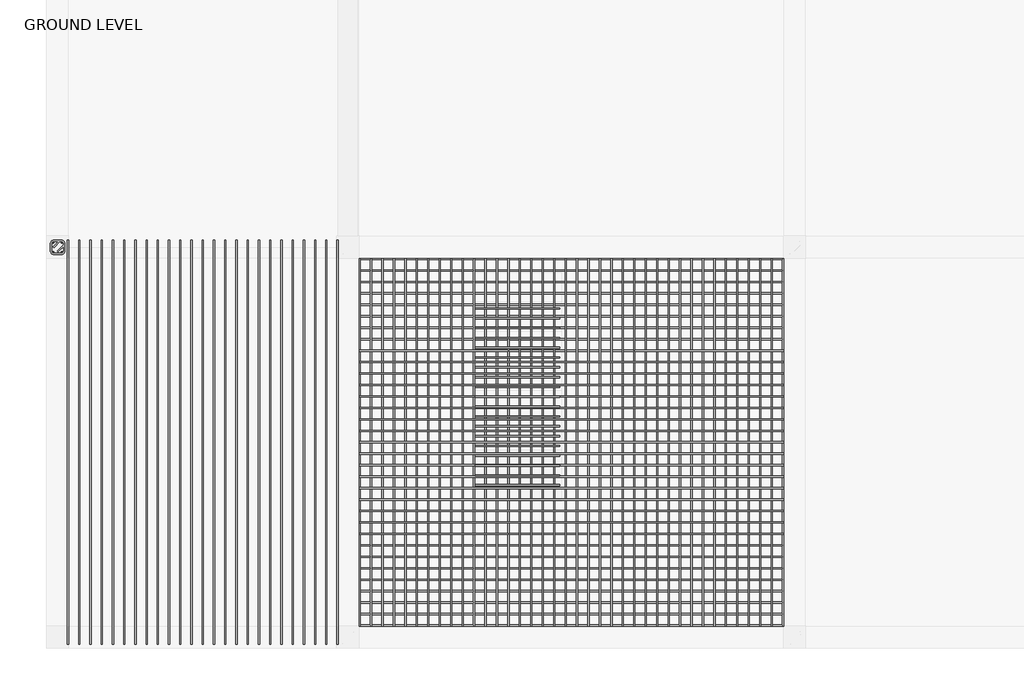
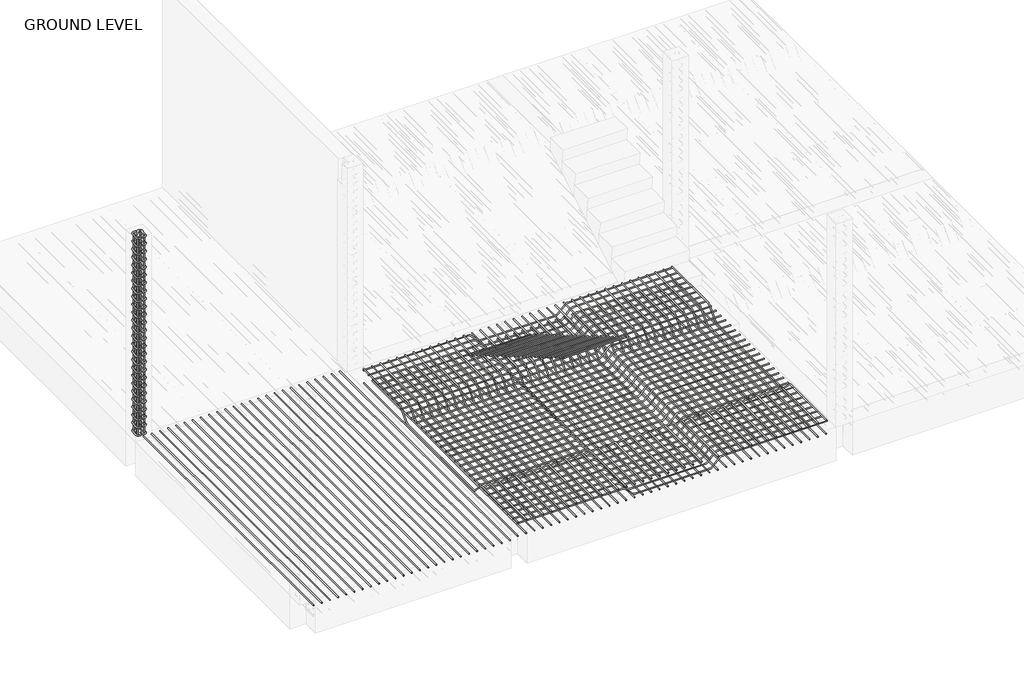
# One storey, part 3 of 8: 8 reinforcing bars.
"""IFC4 building model written with IfcOpenShell, lengths in millimetres."""

from ifc_helpers import new_model, si_unit, point, frame, origin, place, context, project, spatial, polyline, circle_curve, trimmed, segment, composite_curve, source, transform, mapped, element, save
from ifc_brep_helpers import swept_disk

model = new_model("IFC4")

# Units and contexts
model_context = context("Model", 3, world=origin())
ifc_project = project(units=[si_unit("LENGTHUNIT", "METRE", prefix="MILLI")], contexts=[model_context])

# Site, building, storey
site = spatial("IfcSite", under=ifc_project)
building = spatial("IfcBuilding", under=site)
storey = spatial("IfcBuildingStorey", under=building, Name="GROUND LEVEL", Elevation=0.0)

# Reinforcing bars
placement = place(None, origin())
reinforcing_bar_shape = source(origin(), model_context, "Body", "SolidModel", [
    swept_disk(composite_curve([segment(polyline([(-11812.2556799, -353.3525279, -46.35), (-10325.9161368, -353.3525279, -46.35)]), True, "CONTINUOUS"), segment(trimmed(circle_curve(frame((-10325.9161368, -353.3525279, -92.7), z_axis=(0.0, 1.0, 0.0), x_axis=(0.0, 0.0, 46.35)), 46.35), [point((-10325.9161368, -353.3525279, -46.35))], [point((-10293.1417375, -353.3525279, -59.9256007))], True, "CARTESIAN"), True, "CONTINUOUS"), segment(polyline([(-10293.1417375, -353.3525279, -59.9256007), (-10185.2215826, -353.3525279, -167.8457555)]), True, "CONTINUOUS"), segment(trimmed(circle_curve(frame((-10152.4471833, -353.3525279, -135.0713562), z_axis=(0.0, -1.0000000000000002, 0.0), x_axis=(-32.77439929999855, 0.0, -32.7743993)), 46.35), [point((-10185.2215826, -353.3525279, -167.8457555))], [point((-10152.4471833, -353.3525279, -181.4213562))], True, "CARTESIAN"), True, "CONTINUOUS"), segment(polyline([(-10152.4471833, -353.3525279, -181.4213562), (-9088.5758347, -353.3525279, -181.4213562)]), True, "CONTINUOUS"), segment(trimmed(circle_curve(frame((-9088.5758347, -353.3525279, -135.0713562), z_axis=(0.0, -1.0, 0.0), x_axis=(0.0, 0.0, -46.349999999999994)), 46.35), [point((-9088.5758347, -353.3525279, -181.4213562))], [point((-9055.8014354, -353.3525279, -167.8457555))], True, "CARTESIAN"), True, "CONTINUOUS"), segment(polyline([(-9055.8014354, -353.3525279, -167.8457555), (-8947.8812806, -353.3525279, -59.9256007)]), True, "CONTINUOUS"), segment(trimmed(circle_curve(frame((-8915.1068813, -353.3525279, -92.7), z_axis=(0.0, 1.0000000000000002, 0.0), x_axis=(-32.77439930000037, 0.0, 32.774399300000006)), 46.35), [point((-8947.8812806, -353.3525279, -59.9256007))], [point((-8915.1068813, -353.3525279, -46.35))], True, "CARTESIAN"), True, "CONTINUOUS"), segment(polyline([(-8915.1068813, -353.3525279, -46.35), (-7428.7673382, -353.3525279, -46.35)]), True, "CONTINUOUS")], self_intersect=False), 6.35),
])
element("IfcReinforcingBar", 1, at=placement, inside=storey, context=model_context, shape_type="MappedRepresentation", body=[
    mapped(reinforcing_bar_shape, transform((0.0, 0.0, 0.0), x_axis=(1.0, 0.0, 0.0), y_axis=(0.0, 1.0, 0.0), z_axis=(0.0, 0.0, 1.0))),
    mapped(reinforcing_bar_shape, transform((0.0, -118.309244, 0.0), x_axis=(1.0, 0.0, 0.0), y_axis=(0.0, 1.0, 0.0), z_axis=(0.0, 0.0, 1.0))),
    mapped(reinforcing_bar_shape, transform((0.0, -236.6184879, 0.0), x_axis=(1.0, 0.0, 0.0), y_axis=(0.0, 1.0, 0.0), z_axis=(0.0, 0.0, 1.0))),
    mapped(reinforcing_bar_shape, transform((0.0, -354.9277319, 0.0), x_axis=(1.0, 0.0, 0.0), y_axis=(0.0, 1.0, 0.0), z_axis=(0.0, 0.0, 1.0))),
    mapped(reinforcing_bar_shape, transform((0.0, -473.2369759, 0.0), x_axis=(1.0, 0.0, 0.0), y_axis=(0.0, 1.0, 0.0), z_axis=(0.0, 0.0, 1.0))),
    mapped(reinforcing_bar_shape, transform((0.0, -591.5462199, 0.0), x_axis=(1.0, 0.0, 0.0), y_axis=(0.0, 1.0, 0.0), z_axis=(0.0, 0.0, 1.0))),
    mapped(reinforcing_bar_shape, transform((0.0, -709.8554638, 0.0), x_axis=(1.0, 0.0, 0.0), y_axis=(0.0, 1.0, 0.0), z_axis=(0.0, 0.0, 1.0))),
    mapped(reinforcing_bar_shape, transform((0.0, -828.1647078, 0.0), x_axis=(1.0, 0.0, 0.0), y_axis=(0.0, 1.0, 0.0), z_axis=(0.0, 0.0, 1.0))),
    mapped(reinforcing_bar_shape, transform((0.0, -946.4739518, 0.0), x_axis=(1.0, 0.0, 0.0), y_axis=(0.0, 1.0, 0.0), z_axis=(0.0, 0.0, 1.0))),
    mapped(reinforcing_bar_shape, transform((0.0, -1064.7831957, 0.0), x_axis=(1.0, 0.0, 0.0), y_axis=(0.0, 1.0, 0.0), z_axis=(0.0, 0.0, 1.0))),
    mapped(reinforcing_bar_shape, transform((0.0, -1183.0924397, 0.0), x_axis=(1.0, 0.0, 0.0), y_axis=(0.0, 1.0, 0.0), z_axis=(0.0, 0.0, 1.0))),
    mapped(reinforcing_bar_shape, transform((0.0, -1301.4016837, 0.0), x_axis=(1.0, 0.0, 0.0), y_axis=(0.0, 1.0, 0.0), z_axis=(0.0, 0.0, 1.0))),
    mapped(reinforcing_bar_shape, transform((0.0, -1419.7109276, 0.0), x_axis=(1.0, 0.0, 0.0), y_axis=(0.0, 1.0, 0.0), z_axis=(0.0, 0.0, 1.0))),
    mapped(reinforcing_bar_shape, transform((0.0, -1538.0201716, 0.0), x_axis=(1.0, 0.0, 0.0), y_axis=(0.0, 1.0, 0.0), z_axis=(0.0, 0.0, 1.0))),
    mapped(reinforcing_bar_shape, transform((0.0, -1656.3294156, 0.0), x_axis=(1.0, 0.0, 0.0), y_axis=(0.0, 1.0, 0.0), z_axis=(0.0, 0.0, 1.0))),
    mapped(reinforcing_bar_shape, transform((0.0, -1774.6386596, 0.0), x_axis=(1.0, 0.0, 0.0), y_axis=(0.0, 1.0, 0.0), z_axis=(0.0, 0.0, 1.0))),
    mapped(reinforcing_bar_shape, transform((0.0, -1892.9479035, 0.0), x_axis=(1.0, 0.0, 0.0), y_axis=(0.0, 1.0, 0.0), z_axis=(0.0, 0.0, 1.0))),
    mapped(reinforcing_bar_shape, transform((0.0, -2011.2571475, 0.0), x_axis=(1.0, 0.0, 0.0), y_axis=(0.0, 1.0, 0.0), z_axis=(0.0, 0.0, 1.0))),
    mapped(reinforcing_bar_shape, transform((0.0, -2129.5663915, 0.0), x_axis=(1.0, 0.0, 0.0), y_axis=(0.0, 1.0, 0.0), z_axis=(0.0, 0.0, 1.0))),
    mapped(reinforcing_bar_shape, transform((0.0, -2247.8756354, 0.0), x_axis=(1.0, 0.0, 0.0), y_axis=(0.0, 1.0, 0.0), z_axis=(0.0, 0.0, 1.0))),
    mapped(reinforcing_bar_shape, transform((0.0, -2366.1848794, 0.0), x_axis=(1.0, 0.0, 0.0), y_axis=(0.0, 1.0, 0.0), z_axis=(0.0, 0.0, 1.0))),
    mapped(reinforcing_bar_shape, transform((0.0, -2484.4941234, 0.0), x_axis=(1.0, 0.0, 0.0), y_axis=(0.0, 1.0, 0.0), z_axis=(0.0, 0.0, 1.0))),
    mapped(reinforcing_bar_shape, transform((0.0, -2602.8033673, 0.0), x_axis=(1.0, 0.0, 0.0), y_axis=(0.0, 1.0, 0.0), z_axis=(0.0, 0.0, 1.0))),
    mapped(reinforcing_bar_shape, transform((0.0, -2721.1126113, 0.0), x_axis=(1.0, 0.0, 0.0), y_axis=(0.0, 1.0, 0.0), z_axis=(0.0, 0.0, 1.0))),
    mapped(reinforcing_bar_shape, transform((0.0, -2839.4218553, 0.0), x_axis=(1.0, 0.0, 0.0), y_axis=(0.0, 1.0, 0.0), z_axis=(0.0, 0.0, 1.0))),
    mapped(reinforcing_bar_shape, transform((0.0, -2957.7310993, 0.0), x_axis=(1.0, 0.0, 0.0), y_axis=(0.0, 1.0, 0.0), z_axis=(0.0, 0.0, 1.0))),
    mapped(reinforcing_bar_shape, transform((0.0, -3076.0403432, 0.0), x_axis=(1.0, 0.0, 0.0), y_axis=(0.0, 1.0, 0.0), z_axis=(0.0, 0.0, 1.0))),
    mapped(reinforcing_bar_shape, transform((0.0, -3194.3495872, 0.0), x_axis=(1.0, 0.0, 0.0), y_axis=(0.0, 1.0, 0.0), z_axis=(0.0, 0.0, 1.0))),
    mapped(reinforcing_bar_shape, transform((0.0, -3312.6588312, 0.0), x_axis=(1.0, 0.0, 0.0), y_axis=(0.0, 1.0, 0.0), z_axis=(0.0, 0.0, 1.0))),
    mapped(reinforcing_bar_shape, transform((0.0, -3430.9680751, 0.0), x_axis=(1.0, 0.0, 0.0), y_axis=(0.0, 1.0, 0.0), z_axis=(0.0, 0.0, 1.0))),
    mapped(reinforcing_bar_shape, transform((0.0, -3549.2773191, 0.0), x_axis=(1.0, 0.0, 0.0), y_axis=(0.0, 1.0, 0.0), z_axis=(0.0, 0.0, 1.0))),
    mapped(reinforcing_bar_shape, transform((0.0, -3667.5865631, 0.0), x_axis=(1.0, 0.0, 0.0), y_axis=(0.0, 1.0, 0.0), z_axis=(0.0, 0.0, 1.0))),
    mapped(reinforcing_bar_shape, transform((0.0, -3785.895807, 0.0), x_axis=(1.0, 0.0, 0.0), y_axis=(0.0, 1.0, 0.0), z_axis=(0.0, 0.0, 1.0))),
])
reinforcing_bar_2_shape = source(origin(), model_context, "Body", "SolidModel", [
    swept_disk(composite_curve([segment(polyline([(-7435.1173382, -347.0025279, -31.8755724), (-7435.1173382, -1227.8037293, -31.8755724)]), True, "CONTINUOUS"), segment(trimmed(circle_curve(frame((-7435.1173382, -1227.8037293, -78.2255724), z_axis=(1.0, 0.0, 0.0), x_axis=(0.0, 0.0, 46.35000000000001)), 46.35), [point((-7435.1173382, -1227.8037293, -31.8755724))], [point((-7435.1173382, -1260.5781286, -45.4511731))], True, "CARTESIAN"), True, "CONTINUOUS"), segment(polyline([(-7435.1173382, -1260.5781286, -45.4511731), (-7435.1173382, -1410.9101229, -195.7831675)]), True, "CONTINUOUS"), segment(trimmed(circle_curve(frame((-7435.1173382, -1443.6845222, -163.0087682), z_axis=(-1.0, 0.0, 0.0), x_axis=(0.0, 32.774399299999914, -32.7743993)), 46.35), [point((-7435.1173382, -1410.9101229, -195.7831675))], [point((-7435.1173382, -1443.6845222, -209.3587682))], True, "CARTESIAN"), True, "CONTINUOUS"), segment(polyline([(-7435.1173382, -1443.6845222, -209.3587682), (-7435.1173382, -3048.9163406, -209.3587682)]), True, "CONTINUOUS"), segment(trimmed(circle_curve(frame((-7435.1173382, -3048.9163406, -163.0087682), z_axis=(-1.0, 0.0, 0.0), x_axis=(0.0, 0.0, -46.349999999999994)), 46.35), [point((-7435.1173382, -3048.9163406, -209.3587682))], [point((-7435.1173382, -3081.6907399, -195.7831675))], True, "CARTESIAN"), True, "CONTINUOUS"), segment(polyline([(-7435.1173382, -3081.6907399, -195.7831675), (-7435.1173382, -3232.0227342, -45.4511731)]), True, "CONTINUOUS"), segment(trimmed(circle_curve(frame((-7435.1173382, -3264.7971335, -78.2255724), z_axis=(1.0, 0.0, 0.0), x_axis=(0.0, 32.77439930000037, 32.774399300000006)), 46.35), [point((-7435.1173382, -3232.0227342, -45.4511731))], [point((-7435.1173382, -3264.7971335, -31.8755724))], True, "CARTESIAN"), True, "CONTINUOUS"), segment(polyline([(-7435.1173382, -3264.7971335, -31.8755724), (-7435.1173382, -4145.5983349, -31.8755724)]), True, "CONTINUOUS")], self_intersect=False), 6.35),
])
element("IfcReinforcingBar", 2, at=placement, inside=storey, context=model_context, shape_type="MappedRepresentation", body=[
    mapped(reinforcing_bar_2_shape, transform((0.0, 0.0, 0.0), x_axis=(1.0, 0.0, 0.0), y_axis=(0.0, 1.0, 0.0), z_axis=(0.0, 0.0, 1.0))),
    mapped(reinforcing_bar_2_shape, transform((-118.1294146, 0.0, 0.0), x_axis=(1.0, 0.0, 0.0), y_axis=(0.0, 1.0, 0.0), z_axis=(0.0, 0.0, 1.0))),
    mapped(reinforcing_bar_2_shape, transform((-236.2588293, 0.0, 0.0), x_axis=(1.0, 0.0, 0.0), y_axis=(0.0, 1.0, 0.0), z_axis=(0.0, 0.0, 1.0))),
    mapped(reinforcing_bar_2_shape, transform((-354.3882439, 0.0, 0.0), x_axis=(1.0, 0.0, 0.0), y_axis=(0.0, 1.0, 0.0), z_axis=(0.0, 0.0, 1.0))),
    mapped(reinforcing_bar_2_shape, transform((-472.5176586, 0.0, 0.0), x_axis=(1.0, 0.0, 0.0), y_axis=(0.0, 1.0, 0.0), z_axis=(0.0, 0.0, 1.0))),
    mapped(reinforcing_bar_2_shape, transform((-590.6470732, 0.0, 0.0), x_axis=(1.0, 0.0, 0.0), y_axis=(0.0, 1.0, 0.0), z_axis=(0.0, 0.0, 1.0))),
    mapped(reinforcing_bar_2_shape, transform((-708.7764878, 0.0, 0.0), x_axis=(1.0, 0.0, 0.0), y_axis=(0.0, 1.0, 0.0), z_axis=(0.0, 0.0, 1.0))),
    mapped(reinforcing_bar_2_shape, transform((-826.9059025, 0.0, 0.0), x_axis=(1.0, 0.0, 0.0), y_axis=(0.0, 1.0, 0.0), z_axis=(0.0, 0.0, 1.0))),
    mapped(reinforcing_bar_2_shape, transform((-945.0353171, 0.0, 0.0), x_axis=(1.0, 0.0, 0.0), y_axis=(0.0, 1.0, 0.0), z_axis=(0.0, 0.0, 1.0))),
    mapped(reinforcing_bar_2_shape, transform((-1063.1647318, 0.0, 0.0), x_axis=(1.0, 0.0, 0.0), y_axis=(0.0, 1.0, 0.0), z_axis=(0.0, 0.0, 1.0))),
    mapped(reinforcing_bar_2_shape, transform((-1181.2941464, 0.0, 0.0), x_axis=(1.0, 0.0, 0.0), y_axis=(0.0, 1.0, 0.0), z_axis=(0.0, 0.0, 1.0))),
    mapped(reinforcing_bar_2_shape, transform((-1299.423561, 0.0, 0.0), x_axis=(1.0, 0.0, 0.0), y_axis=(0.0, 1.0, 0.0), z_axis=(0.0, 0.0, 1.0))),
    mapped(reinforcing_bar_2_shape, transform((-1417.5529757, 0.0, 0.0), x_axis=(1.0, 0.0, 0.0), y_axis=(0.0, 1.0, 0.0), z_axis=(0.0, 0.0, 1.0))),
    mapped(reinforcing_bar_2_shape, transform((-1535.6823903, 0.0, 0.0), x_axis=(1.0, 0.0, 0.0), y_axis=(0.0, 1.0, 0.0), z_axis=(0.0, 0.0, 1.0))),
    mapped(reinforcing_bar_2_shape, transform((-1653.811805, 0.0, 0.0), x_axis=(1.0, 0.0, 0.0), y_axis=(0.0, 1.0, 0.0), z_axis=(0.0, 0.0, 1.0))),
    mapped(reinforcing_bar_2_shape, transform((-1771.9412196, 0.0, 0.0), x_axis=(1.0, 0.0, 0.0), y_axis=(0.0, 1.0, 0.0), z_axis=(0.0, 0.0, 1.0))),
    mapped(reinforcing_bar_2_shape, transform((-1890.0706342, 0.0, 0.0), x_axis=(1.0, 0.0, 0.0), y_axis=(0.0, 1.0, 0.0), z_axis=(0.0, 0.0, 1.0))),
    mapped(reinforcing_bar_2_shape, transform((-2008.2000489, 0.0, 0.0), x_axis=(1.0, 0.0, 0.0), y_axis=(0.0, 1.0, 0.0), z_axis=(0.0, 0.0, 1.0))),
    mapped(reinforcing_bar_2_shape, transform((-2126.3294635, 0.0, 0.0), x_axis=(1.0, 0.0, 0.0), y_axis=(0.0, 1.0, 0.0), z_axis=(0.0, 0.0, 1.0))),
    mapped(reinforcing_bar_2_shape, transform((-2244.4588782, 0.0, 0.0), x_axis=(1.0, 0.0, 0.0), y_axis=(0.0, 1.0, 0.0), z_axis=(0.0, 0.0, 1.0))),
    mapped(reinforcing_bar_2_shape, transform((-2362.5882928, 0.0, 0.0), x_axis=(1.0, 0.0, 0.0), y_axis=(0.0, 1.0, 0.0), z_axis=(0.0, 0.0, 1.0))),
    mapped(reinforcing_bar_2_shape, transform((-2480.7177075, 0.0, 0.0), x_axis=(1.0, 0.0, 0.0), y_axis=(0.0, 1.0, 0.0), z_axis=(0.0, 0.0, 1.0))),
    mapped(reinforcing_bar_2_shape, transform((-2598.8471221, 0.0, 0.0), x_axis=(1.0, 0.0, 0.0), y_axis=(0.0, 1.0, 0.0), z_axis=(0.0, 0.0, 1.0))),
    mapped(reinforcing_bar_2_shape, transform((-2716.9765367, 0.0, 0.0), x_axis=(1.0, 0.0, 0.0), y_axis=(0.0, 1.0, 0.0), z_axis=(0.0, 0.0, 1.0))),
    mapped(reinforcing_bar_2_shape, transform((-2835.1059514, 0.0, 0.0), x_axis=(1.0, 0.0, 0.0), y_axis=(0.0, 1.0, 0.0), z_axis=(0.0, 0.0, 1.0))),
    mapped(reinforcing_bar_2_shape, transform((-2953.235366, 0.0, 0.0), x_axis=(1.0, 0.0, 0.0), y_axis=(0.0, 1.0, 0.0), z_axis=(0.0, 0.0, 1.0))),
    mapped(reinforcing_bar_2_shape, transform((-3071.3647807, 0.0, 0.0), x_axis=(1.0, 0.0, 0.0), y_axis=(0.0, 1.0, 0.0), z_axis=(0.0, 0.0, 1.0))),
    mapped(reinforcing_bar_2_shape, transform((-3189.4941953, 0.0, 0.0), x_axis=(1.0, 0.0, 0.0), y_axis=(0.0, 1.0, 0.0), z_axis=(0.0, 0.0, 1.0))),
    mapped(reinforcing_bar_2_shape, transform((-3307.6236099, 0.0, 0.0), x_axis=(1.0, 0.0, 0.0), y_axis=(0.0, 1.0, 0.0), z_axis=(0.0, 0.0, 1.0))),
    mapped(reinforcing_bar_2_shape, transform((-3425.7530246, 0.0, 0.0), x_axis=(1.0, 0.0, 0.0), y_axis=(0.0, 1.0, 0.0), z_axis=(0.0, 0.0, 1.0))),
    mapped(reinforcing_bar_2_shape, transform((-3543.8824392, 0.0, 0.0), x_axis=(1.0, 0.0, 0.0), y_axis=(0.0, 1.0, 0.0), z_axis=(0.0, 0.0, 1.0))),
    mapped(reinforcing_bar_2_shape, transform((-3662.0118539, 0.0, 0.0), x_axis=(1.0, 0.0, 0.0), y_axis=(0.0, 1.0, 0.0), z_axis=(0.0, 0.0, 1.0))),
    mapped(reinforcing_bar_2_shape, transform((-3780.1412685, 0.0, 0.0), x_axis=(1.0, 0.0, 0.0), y_axis=(0.0, 1.0, 0.0), z_axis=(0.0, 0.0, 1.0))),
    mapped(reinforcing_bar_2_shape, transform((-3898.2706831, 0.0, 0.0), x_axis=(1.0, 0.0, 0.0), y_axis=(0.0, 1.0, 0.0), z_axis=(0.0, 0.0, 1.0))),
    mapped(reinforcing_bar_2_shape, transform((-4016.4000978, 0.0, 0.0), x_axis=(1.0, 0.0, 0.0), y_axis=(0.0, 1.0, 0.0), z_axis=(0.0, 0.0, 1.0))),
    mapped(reinforcing_bar_2_shape, transform((-4134.5295124, 0.0, 0.0), x_axis=(1.0, 0.0, 0.0), y_axis=(0.0, 1.0, 0.0), z_axis=(0.0, 0.0, 1.0))),
    mapped(reinforcing_bar_2_shape, transform((-4252.6589271, 0.0, 0.0), x_axis=(1.0, 0.0, 0.0), y_axis=(0.0, 1.0, 0.0), z_axis=(0.0, 0.0, 1.0))),
    mapped(reinforcing_bar_2_shape, transform((-4370.7883417, 0.0, 0.0), x_axis=(1.0, 0.0, 0.0), y_axis=(0.0, 1.0, 0.0), z_axis=(0.0, 0.0, 1.0))),
])
reinforcing_bar_3_shape = source(origin(), model_context, "Body", "SolidModel", [
    swept_disk(composite_curve([segment(polyline([(-7435.1173382, -4134.0810507, -240.830741), (-7435.1173382, -358.1289151, -240.830741)]), True, "CONTINUOUS")], self_intersect=False), 6.35),
])
element("IfcReinforcingBar", 3, at=placement, inside=storey, context=model_context, shape_type="MappedRepresentation", body=[
    mapped(reinforcing_bar_3_shape, transform((0.0, 0.0, 0.0), x_axis=(1.0, 0.0, 0.0), y_axis=(0.0, 1.0, 0.0), z_axis=(0.0, 0.0, 1.0))),
    mapped(reinforcing_bar_3_shape, transform((-118.1294146, 0.0, 0.0), x_axis=(1.0, 0.0, 0.0), y_axis=(0.0, 1.0, 0.0), z_axis=(0.0, 0.0, 1.0))),
    mapped(reinforcing_bar_3_shape, transform((-236.2588293, 0.0, 0.0), x_axis=(1.0, 0.0, 0.0), y_axis=(0.0, 1.0, 0.0), z_axis=(0.0, 0.0, 1.0))),
    mapped(reinforcing_bar_3_shape, transform((-354.3882439, 0.0, 0.0), x_axis=(1.0, 0.0, 0.0), y_axis=(0.0, 1.0, 0.0), z_axis=(0.0, 0.0, 1.0))),
    mapped(reinforcing_bar_3_shape, transform((-472.5176586, 0.0, 0.0), x_axis=(1.0, 0.0, 0.0), y_axis=(0.0, 1.0, 0.0), z_axis=(0.0, 0.0, 1.0))),
    mapped(reinforcing_bar_3_shape, transform((-590.6470732, 0.0, 0.0), x_axis=(1.0, 0.0, 0.0), y_axis=(0.0, 1.0, 0.0), z_axis=(0.0, 0.0, 1.0))),
    mapped(reinforcing_bar_3_shape, transform((-708.7764878, 0.0, 0.0), x_axis=(1.0, 0.0, 0.0), y_axis=(0.0, 1.0, 0.0), z_axis=(0.0, 0.0, 1.0))),
    mapped(reinforcing_bar_3_shape, transform((-826.9059025, 0.0, 0.0), x_axis=(1.0, 0.0, 0.0), y_axis=(0.0, 1.0, 0.0), z_axis=(0.0, 0.0, 1.0))),
    mapped(reinforcing_bar_3_shape, transform((-945.0353171, 0.0, 0.0), x_axis=(1.0, 0.0, 0.0), y_axis=(0.0, 1.0, 0.0), z_axis=(0.0, 0.0, 1.0))),
    mapped(reinforcing_bar_3_shape, transform((-1063.1647318, 0.0, 0.0), x_axis=(1.0, 0.0, 0.0), y_axis=(0.0, 1.0, 0.0), z_axis=(0.0, 0.0, 1.0))),
    mapped(reinforcing_bar_3_shape, transform((-1181.2941464, 0.0, 0.0), x_axis=(1.0, 0.0, 0.0), y_axis=(0.0, 1.0, 0.0), z_axis=(0.0, 0.0, 1.0))),
    mapped(reinforcing_bar_3_shape, transform((-1299.423561, 0.0, 0.0), x_axis=(1.0, 0.0, 0.0), y_axis=(0.0, 1.0, 0.0), z_axis=(0.0, 0.0, 1.0))),
    mapped(reinforcing_bar_3_shape, transform((-1417.5529757, 0.0, 0.0), x_axis=(1.0, 0.0, 0.0), y_axis=(0.0, 1.0, 0.0), z_axis=(0.0, 0.0, 1.0))),
    mapped(reinforcing_bar_3_shape, transform((-1535.6823903, 0.0, 0.0), x_axis=(1.0, 0.0, 0.0), y_axis=(0.0, 1.0, 0.0), z_axis=(0.0, 0.0, 1.0))),
    mapped(reinforcing_bar_3_shape, transform((-1653.811805, 0.0, 0.0), x_axis=(1.0, 0.0, 0.0), y_axis=(0.0, 1.0, 0.0), z_axis=(0.0, 0.0, 1.0))),
    mapped(reinforcing_bar_3_shape, transform((-1771.9412196, 0.0, 0.0), x_axis=(1.0, 0.0, 0.0), y_axis=(0.0, 1.0, 0.0), z_axis=(0.0, 0.0, 1.0))),
    mapped(reinforcing_bar_3_shape, transform((-1890.0706342, 0.0, 0.0), x_axis=(1.0, 0.0, 0.0), y_axis=(0.0, 1.0, 0.0), z_axis=(0.0, 0.0, 1.0))),
    mapped(reinforcing_bar_3_shape, transform((-2008.2000489, 0.0, 0.0), x_axis=(1.0, 0.0, 0.0), y_axis=(0.0, 1.0, 0.0), z_axis=(0.0, 0.0, 1.0))),
    mapped(reinforcing_bar_3_shape, transform((-2126.3294635, 0.0, 0.0), x_axis=(1.0, 0.0, 0.0), y_axis=(0.0, 1.0, 0.0), z_axis=(0.0, 0.0, 1.0))),
    mapped(reinforcing_bar_3_shape, transform((-2244.4588782, 0.0, 0.0), x_axis=(1.0, 0.0, 0.0), y_axis=(0.0, 1.0, 0.0), z_axis=(0.0, 0.0, 1.0))),
    mapped(reinforcing_bar_3_shape, transform((-2362.5882928, 0.0, 0.0), x_axis=(1.0, 0.0, 0.0), y_axis=(0.0, 1.0, 0.0), z_axis=(0.0, 0.0, 1.0))),
    mapped(reinforcing_bar_3_shape, transform((-2480.7177075, 0.0, 0.0), x_axis=(1.0, 0.0, 0.0), y_axis=(0.0, 1.0, 0.0), z_axis=(0.0, 0.0, 1.0))),
    mapped(reinforcing_bar_3_shape, transform((-2598.8471221, 0.0, 0.0), x_axis=(1.0, 0.0, 0.0), y_axis=(0.0, 1.0, 0.0), z_axis=(0.0, 0.0, 1.0))),
    mapped(reinforcing_bar_3_shape, transform((-2716.9765367, 0.0, 0.0), x_axis=(1.0, 0.0, 0.0), y_axis=(0.0, 1.0, 0.0), z_axis=(0.0, 0.0, 1.0))),
    mapped(reinforcing_bar_3_shape, transform((-2835.1059514, 0.0, 0.0), x_axis=(1.0, 0.0, 0.0), y_axis=(0.0, 1.0, 0.0), z_axis=(0.0, 0.0, 1.0))),
    mapped(reinforcing_bar_3_shape, transform((-2953.235366, 0.0, 0.0), x_axis=(1.0, 0.0, 0.0), y_axis=(0.0, 1.0, 0.0), z_axis=(0.0, 0.0, 1.0))),
    mapped(reinforcing_bar_3_shape, transform((-3071.3647807, 0.0, 0.0), x_axis=(1.0, 0.0, 0.0), y_axis=(0.0, 1.0, 0.0), z_axis=(0.0, 0.0, 1.0))),
    mapped(reinforcing_bar_3_shape, transform((-3189.4941953, 0.0, 0.0), x_axis=(1.0, 0.0, 0.0), y_axis=(0.0, 1.0, 0.0), z_axis=(0.0, 0.0, 1.0))),
    mapped(reinforcing_bar_3_shape, transform((-3307.6236099, 0.0, 0.0), x_axis=(1.0, 0.0, 0.0), y_axis=(0.0, 1.0, 0.0), z_axis=(0.0, 0.0, 1.0))),
    mapped(reinforcing_bar_3_shape, transform((-3425.7530246, 0.0, 0.0), x_axis=(1.0, 0.0, 0.0), y_axis=(0.0, 1.0, 0.0), z_axis=(0.0, 0.0, 1.0))),
    mapped(reinforcing_bar_3_shape, transform((-3543.8824392, 0.0, 0.0), x_axis=(1.0, 0.0, 0.0), y_axis=(0.0, 1.0, 0.0), z_axis=(0.0, 0.0, 1.0))),
    mapped(reinforcing_bar_3_shape, transform((-3662.0118539, 0.0, 0.0), x_axis=(1.0, 0.0, 0.0), y_axis=(0.0, 1.0, 0.0), z_axis=(0.0, 0.0, 1.0))),
    mapped(reinforcing_bar_3_shape, transform((-3780.1412685, 0.0, 0.0), x_axis=(1.0, 0.0, 0.0), y_axis=(0.0, 1.0, 0.0), z_axis=(0.0, 0.0, 1.0))),
    mapped(reinforcing_bar_3_shape, transform((-3898.2706831, 0.0, 0.0), x_axis=(1.0, 0.0, 0.0), y_axis=(0.0, 1.0, 0.0), z_axis=(0.0, 0.0, 1.0))),
    mapped(reinforcing_bar_3_shape, transform((-4016.4000978, 0.0, 0.0), x_axis=(1.0, 0.0, 0.0), y_axis=(0.0, 1.0, 0.0), z_axis=(0.0, 0.0, 1.0))),
    mapped(reinforcing_bar_3_shape, transform((-4134.5295124, 0.0, 0.0), x_axis=(1.0, 0.0, 0.0), y_axis=(0.0, 1.0, 0.0), z_axis=(0.0, 0.0, 1.0))),
    mapped(reinforcing_bar_3_shape, transform((-4252.6589271, 0.0, 0.0), x_axis=(1.0, 0.0, 0.0), y_axis=(0.0, 1.0, 0.0), z_axis=(0.0, 0.0, 1.0))),
    mapped(reinforcing_bar_3_shape, transform((-4370.7883417, 0.0, 0.0), x_axis=(1.0, 0.0, 0.0), y_axis=(0.0, 1.0, 0.0), z_axis=(0.0, 0.0, 1.0))),
])
reinforcing_bar_4_shape = source(origin(), model_context, "Body", "SolidModel", [
    swept_disk(composite_curve([segment(polyline([(-14816.7556793, -158.4025279, -105.2544844), (-14816.7556793, -4334.1983349, -105.2544844)]), True, "CONTINUOUS")], self_intersect=False), 6.35),
])
element("IfcReinforcingBar", 4, at=placement, inside=storey, context=model_context, shape_type="MappedRepresentation", body=[
    mapped(reinforcing_bar_4_shape, transform((0.0, 0.0, 0.0), x_axis=(1.0, 0.0, 0.0), y_axis=(0.0, 1.0, 0.0), z_axis=(0.0, 0.0, 1.0))),
    mapped(reinforcing_bar_4_shape, transform((115.9666666, 0.0, 0.0), x_axis=(1.0, 0.0, 0.0), y_axis=(0.0, 1.0, 0.0), z_axis=(0.0, 0.0, 1.0))),
    mapped(reinforcing_bar_4_shape, transform((231.9333332, 0.0, 0.0), x_axis=(1.0, 0.0, 0.0), y_axis=(0.0, 1.0, 0.0), z_axis=(0.0, 0.0, 1.0))),
    mapped(reinforcing_bar_4_shape, transform((347.8999998, 0.0, 0.0), x_axis=(1.0, 0.0, 0.0), y_axis=(0.0, 1.0, 0.0), z_axis=(0.0, 0.0, 1.0))),
    mapped(reinforcing_bar_4_shape, transform((463.8666665, 0.0, 0.0), x_axis=(1.0, 0.0, 0.0), y_axis=(0.0, 1.0, 0.0), z_axis=(0.0, 0.0, 1.0))),
    mapped(reinforcing_bar_4_shape, transform((579.8333331, 0.0, 0.0), x_axis=(1.0, 0.0, 0.0), y_axis=(0.0, 1.0, 0.0), z_axis=(0.0, 0.0, 1.0))),
    mapped(reinforcing_bar_4_shape, transform((695.7999997, 0.0, 0.0), x_axis=(1.0, 0.0, 0.0), y_axis=(0.0, 1.0, 0.0), z_axis=(0.0, 0.0, 1.0))),
    mapped(reinforcing_bar_4_shape, transform((811.7666663, 0.0, 0.0), x_axis=(1.0, 0.0, 0.0), y_axis=(0.0, 1.0, 0.0), z_axis=(0.0, 0.0, 1.0))),
    mapped(reinforcing_bar_4_shape, transform((927.7333329, 0.0, 0.0), x_axis=(1.0, 0.0, 0.0), y_axis=(0.0, 1.0, 0.0), z_axis=(0.0, 0.0, 1.0))),
    mapped(reinforcing_bar_4_shape, transform((1043.6999995, 0.0, 0.0), x_axis=(1.0, 0.0, 0.0), y_axis=(0.0, 1.0, 0.0), z_axis=(0.0, 0.0, 1.0))),
    mapped(reinforcing_bar_4_shape, transform((1159.6666662, 0.0, 0.0), x_axis=(1.0, 0.0, 0.0), y_axis=(0.0, 1.0, 0.0), z_axis=(0.0, 0.0, 1.0))),
    mapped(reinforcing_bar_4_shape, transform((1275.6333328, 0.0, 0.0), x_axis=(1.0, 0.0, 0.0), y_axis=(0.0, 1.0, 0.0), z_axis=(0.0, 0.0, 1.0))),
    mapped(reinforcing_bar_4_shape, transform((1391.5999994, 0.0, 0.0), x_axis=(1.0, 0.0, 0.0), y_axis=(0.0, 1.0, 0.0), z_axis=(0.0, 0.0, 1.0))),
    mapped(reinforcing_bar_4_shape, transform((1507.566666, 0.0, 0.0), x_axis=(1.0, 0.0, 0.0), y_axis=(0.0, 1.0, 0.0), z_axis=(0.0, 0.0, 1.0))),
    mapped(reinforcing_bar_4_shape, transform((1623.5333326, 0.0, 0.0), x_axis=(1.0, 0.0, 0.0), y_axis=(0.0, 1.0, 0.0), z_axis=(0.0, 0.0, 1.0))),
    mapped(reinforcing_bar_4_shape, transform((1739.4999992, 0.0, 0.0), x_axis=(1.0, 0.0, 0.0), y_axis=(0.0, 1.0, 0.0), z_axis=(0.0, 0.0, 1.0))),
    mapped(reinforcing_bar_4_shape, transform((1855.4666659, 0.0, 0.0), x_axis=(1.0, 0.0, 0.0), y_axis=(0.0, 1.0, 0.0), z_axis=(0.0, 0.0, 1.0))),
    mapped(reinforcing_bar_4_shape, transform((1971.4333325, 0.0, 0.0), x_axis=(1.0, 0.0, 0.0), y_axis=(0.0, 1.0, 0.0), z_axis=(0.0, 0.0, 1.0))),
    mapped(reinforcing_bar_4_shape, transform((2087.3999991, 0.0, 0.0), x_axis=(1.0, 0.0, 0.0), y_axis=(0.0, 1.0, 0.0), z_axis=(0.0, 0.0, 1.0))),
    mapped(reinforcing_bar_4_shape, transform((2203.3666657, 0.0, 0.0), x_axis=(1.0, 0.0, 0.0), y_axis=(0.0, 1.0, 0.0), z_axis=(0.0, 0.0, 1.0))),
    mapped(reinforcing_bar_4_shape, transform((2319.3333323, 0.0, 0.0), x_axis=(1.0, 0.0, 0.0), y_axis=(0.0, 1.0, 0.0), z_axis=(0.0, 0.0, 1.0))),
    mapped(reinforcing_bar_4_shape, transform((2435.2999989, 0.0, 0.0), x_axis=(1.0, 0.0, 0.0), y_axis=(0.0, 1.0, 0.0), z_axis=(0.0, 0.0, 1.0))),
    mapped(reinforcing_bar_4_shape, transform((2551.2666655, 0.0, 0.0), x_axis=(1.0, 0.0, 0.0), y_axis=(0.0, 1.0, 0.0), z_axis=(0.0, 0.0, 1.0))),
    mapped(reinforcing_bar_4_shape, transform((2667.2333322, 0.0, 0.0), x_axis=(1.0, 0.0, 0.0), y_axis=(0.0, 1.0, 0.0), z_axis=(0.0, 0.0, 1.0))),
    mapped(reinforcing_bar_4_shape, transform((2783.1999988, 0.0, 0.0), x_axis=(1.0, 0.0, 0.0), y_axis=(0.0, 1.0, 0.0), z_axis=(0.0, 0.0, 1.0))),
])
reinforcing_bar_5_shape = source(origin(), model_context, "Body", "SolidModel", [
    swept_disk(composite_curve([segment(polyline([(-14879.0006936, -183.9048321, 3008.0), (-14879.0006936, -183.9048321, 40.0)]), True, "CONTINUOUS")], self_intersect=False), 6.35),
])
element("IfcReinforcingBar", 5, at=placement, inside=storey, context=model_context, shape_type="MappedRepresentation", body=[
    mapped(reinforcing_bar_5_shape, transform((0.0, 0.0, 0.0), x_axis=(1.0, 0.0, 0.0), y_axis=(0.0, 1.0, 0.0), z_axis=(0.0, 0.0, 1.0))),
    mapped(reinforcing_bar_5_shape, transform((0.0, -96.9916148, 0.0), x_axis=(1.0, 0.0, 0.0), y_axis=(0.0, 1.0, 0.0), z_axis=(0.0, 0.0, 1.0))),
])
reinforcing_bar_6_shape = source(origin(), model_context, "Body", "SolidModel", [
    swept_disk(composite_curve([segment(polyline([(-14965.0670404, -229.6782932, 3001.65), (-14909.3234775, -173.9347303, 3001.65)]), True, "CONTINUOUS"), segment(trimmed(circle_curve(frame((-14887.1556799, -196.1025279, 3001.65), z_axis=(0.0, 0.0, -1.0), x_axis=(-22.167797599999176, 22.1677976, 0.0)), 31.35), [point((-14909.3234775, -173.9347303, 3001.65))], [point((-14855.8056799, -196.1025279, 3001.65))], True, "CARTESIAN"), True, "CONTINUOUS"), segment(polyline([(-14855.8056799, -196.1025279, 3001.65), (-14855.8056799, -269.3025279, 3001.65)]), True, "CONTINUOUS"), segment(trimmed(circle_curve(frame((-14887.1556799, -269.3025279, 3001.65), z_axis=(0.0, 0.0, -1.0), x_axis=(31.350000000000364, 0.0, 0.0)), 31.35), [point((-14855.8056799, -269.3025279, 3001.65))], [point((-14887.1556799, -300.6525279, 3001.65))], True, "CARTESIAN"), True, "CONTINUOUS"), segment(polyline([(-14887.1556799, -300.6525279, 3001.65), (-14960.3556799, -300.6525279, 3001.65)]), True, "CONTINUOUS"), segment(trimmed(circle_curve(frame((-14960.3556799, -269.4385291, 3004.5669815), z_axis=(0.0, 0.09304566152621355, -0.9956618426308951), x_axis=(0.0, -31.213998800000013, -2.91698150000002)), 31.35), [point((-14960.3556799, -300.6525279, 3001.65))], [point((-14991.7056799, -269.4385291, 3004.5669815))], True, "CARTESIAN"), True, "CONTINUOUS"), segment(polyline([(-14991.7056799, -269.4385291, 3004.5669815), (-14991.7056799, -195.9665266, 3011.4330185)]), True, "CONTINUOUS"), segment(trimmed(circle_curve(frame((-14960.3556799, -195.9665266, 3011.4330185), z_axis=(0.0, 0.09304566152621355, -0.9956618426308951), x_axis=(-31.350000000000364, 0.0, 0.0)), 31.35), [point((-14991.7056799, -195.9665266, 3011.4330185))], [point((-14960.3556799, -164.7525279, 3014.35))], True, "CARTESIAN"), True, "CONTINUOUS"), segment(polyline([(-14960.3556799, -164.7525279, 3014.35), (-14887.1556799, -164.7525279, 3014.35)]), True, "CONTINUOUS"), segment(trimmed(circle_curve(frame((-14887.1556799, -196.1025279, 3014.35), z_axis=(0.0, 0.0, -1.0), x_axis=(0.0, 31.350000000000023, 0.0)), 31.35), [point((-14887.1556799, -164.7525279, 3014.35))], [point((-14864.9878823, -218.2703255, 3014.35))], True, "CARTESIAN"), True, "CONTINUOUS"), segment(polyline([(-14864.9878823, -218.2703255, 3014.35), (-14920.7314452, -274.0138884, 3014.35)]), True, "CONTINUOUS")], self_intersect=False), 6.35),
])
element("IfcReinforcingBar", 6, at=placement, inside=storey, context=model_context, shape_type="MappedRepresentation", body=[
    mapped(reinforcing_bar_6_shape, transform((0.0, 0.0, 0.0), x_axis=(1.0, 0.0, 0.0), y_axis=(0.0, 1.0, 0.0), z_axis=(0.0, 0.0, 1.0))),
    mapped(reinforcing_bar_6_shape, transform((0.0, 0.0, -118.212), x_axis=(1.0, 0.0, 0.0), y_axis=(0.0, 1.0, 0.0), z_axis=(0.0, 0.0, 1.0))),
    mapped(reinforcing_bar_6_shape, transform((0.0, 0.0, -236.424), x_axis=(1.0, 0.0, 0.0), y_axis=(0.0, 1.0, 0.0), z_axis=(0.0, 0.0, 1.0))),
    mapped(reinforcing_bar_6_shape, transform((0.0, 0.0, -354.636), x_axis=(1.0, 0.0, 0.0), y_axis=(0.0, 1.0, 0.0), z_axis=(0.0, 0.0, 1.0))),
    mapped(reinforcing_bar_6_shape, transform((0.0, 0.0, -472.848), x_axis=(1.0, 0.0, 0.0), y_axis=(0.0, 1.0, 0.0), z_axis=(0.0, 0.0, 1.0))),
    mapped(reinforcing_bar_6_shape, transform((0.0, 0.0, -591.06), x_axis=(1.0, 0.0, 0.0), y_axis=(0.0, 1.0, 0.0), z_axis=(0.0, 0.0, 1.0))),
    mapped(reinforcing_bar_6_shape, transform((0.0, 0.0, -709.272), x_axis=(1.0, 0.0, 0.0), y_axis=(0.0, 1.0, 0.0), z_axis=(0.0, 0.0, 1.0))),
    mapped(reinforcing_bar_6_shape, transform((0.0, 0.0, -827.484), x_axis=(1.0, 0.0, 0.0), y_axis=(0.0, 1.0, 0.0), z_axis=(0.0, 0.0, 1.0))),
    mapped(reinforcing_bar_6_shape, transform((0.0, 0.0, -945.696), x_axis=(1.0, 0.0, 0.0), y_axis=(0.0, 1.0, 0.0), z_axis=(0.0, 0.0, 1.0))),
    mapped(reinforcing_bar_6_shape, transform((0.0, 0.0, -1063.908), x_axis=(1.0, 0.0, 0.0), y_axis=(0.0, 1.0, 0.0), z_axis=(0.0, 0.0, 1.0))),
    mapped(reinforcing_bar_6_shape, transform((0.0, 0.0, -1182.12), x_axis=(1.0, 0.0, 0.0), y_axis=(0.0, 1.0, 0.0), z_axis=(0.0, 0.0, 1.0))),
    mapped(reinforcing_bar_6_shape, transform((0.0, 0.0, -1300.332), x_axis=(1.0, 0.0, 0.0), y_axis=(0.0, 1.0, 0.0), z_axis=(0.0, 0.0, 1.0))),
    mapped(reinforcing_bar_6_shape, transform((0.0, 0.0, -1418.544), x_axis=(1.0, 0.0, 0.0), y_axis=(0.0, 1.0, 0.0), z_axis=(0.0, 0.0, 1.0))),
    mapped(reinforcing_bar_6_shape, transform((0.0, 0.0, -1536.756), x_axis=(1.0, 0.0, 0.0), y_axis=(0.0, 1.0, 0.0), z_axis=(0.0, 0.0, 1.0))),
    mapped(reinforcing_bar_6_shape, transform((0.0, 0.0, -1654.968), x_axis=(1.0, 0.0, 0.0), y_axis=(0.0, 1.0, 0.0), z_axis=(0.0, 0.0, 1.0))),
    mapped(reinforcing_bar_6_shape, transform((0.0, 0.0, -1773.18), x_axis=(1.0, 0.0, 0.0), y_axis=(0.0, 1.0, 0.0), z_axis=(0.0, 0.0, 1.0))),
    mapped(reinforcing_bar_6_shape, transform((0.0, 0.0, -1891.392), x_axis=(1.0, 0.0, 0.0), y_axis=(0.0, 1.0, 0.0), z_axis=(0.0, 0.0, 1.0))),
    mapped(reinforcing_bar_6_shape, transform((0.0, 0.0, -2009.604), x_axis=(1.0, 0.0, 0.0), y_axis=(0.0, 1.0, 0.0), z_axis=(0.0, 0.0, 1.0))),
    mapped(reinforcing_bar_6_shape, transform((0.0, 0.0, -2127.816), x_axis=(1.0, 0.0, 0.0), y_axis=(0.0, 1.0, 0.0), z_axis=(0.0, 0.0, 1.0))),
    mapped(reinforcing_bar_6_shape, transform((0.0, 0.0, -2246.028), x_axis=(1.0, 0.0, 0.0), y_axis=(0.0, 1.0, 0.0), z_axis=(0.0, 0.0, 1.0))),
    mapped(reinforcing_bar_6_shape, transform((0.0, 0.0, -2364.24), x_axis=(1.0, 0.0, 0.0), y_axis=(0.0, 1.0, 0.0), z_axis=(0.0, 0.0, 1.0))),
    mapped(reinforcing_bar_6_shape, transform((0.0, 0.0, -2482.452), x_axis=(1.0, 0.0, 0.0), y_axis=(0.0, 1.0, 0.0), z_axis=(0.0, 0.0, 1.0))),
    mapped(reinforcing_bar_6_shape, transform((0.0, 0.0, -2600.664), x_axis=(1.0, 0.0, 0.0), y_axis=(0.0, 1.0, 0.0), z_axis=(0.0, 0.0, 1.0))),
    mapped(reinforcing_bar_6_shape, transform((0.0, 0.0, -2718.876), x_axis=(1.0, 0.0, 0.0), y_axis=(0.0, 1.0, 0.0), z_axis=(0.0, 0.0, 1.0))),
    mapped(reinforcing_bar_6_shape, transform((0.0, 0.0, -2837.088), x_axis=(1.0, 0.0, 0.0), y_axis=(0.0, 1.0, 0.0), z_axis=(0.0, 0.0, 1.0))),
    mapped(reinforcing_bar_6_shape, transform((0.0, 0.0, -2955.3), x_axis=(1.0, 0.0, 0.0), y_axis=(0.0, 1.0, 0.0), z_axis=(0.0, 0.0, 1.0))),
])
reinforcing_bar_7_shape = source(origin(), model_context, "Body", "SolidModel", [
    swept_disk(composite_curve([segment(polyline([(-14968.5106662, -183.9048321, 3008.0), (-14968.5106662, -183.9048321, 40.0)]), True, "CONTINUOUS")], self_intersect=False), 6.35),
])
element("IfcReinforcingBar", 7, at=placement, inside=storey, context=model_context, shape_type="MappedRepresentation", body=[
    mapped(reinforcing_bar_7_shape, transform((0.0, 0.0, 0.0), x_axis=(1.0, 0.0, 0.0), y_axis=(0.0, 1.0, 0.0), z_axis=(0.0, 0.0, 1.0))),
    mapped(reinforcing_bar_7_shape, transform((0.0, -96.9916148, 0.0), x_axis=(1.0, 0.0, 0.0), y_axis=(0.0, 1.0, 0.0), z_axis=(0.0, 0.0, 1.0))),
])
reinforcing_bar_8_shape = source(origin(), model_context, "Body", "SolidModel", [
    swept_disk(composite_curve([segment(polyline([(-9739.1476583, -863.4368723, 72.5964632), (-10613.5476583, -863.4368723, 72.5964632)]), True, "CONTINUOUS")], self_intersect=False), 6.35),
])
element("IfcReinforcingBar", 8, at=placement, inside=storey, context=model_context, shape_type="MappedRepresentation", body=[
    mapped(reinforcing_bar_8_shape, transform((0.0, 0.0, 0.0), x_axis=(1.0, 0.0, 0.0), y_axis=(0.0, 1.0, 0.0), z_axis=(0.0, 0.0, 1.0))),
    mapped(reinforcing_bar_8_shape, transform((0.0, -101.5024203, 59.7073061), x_axis=(1.0, 0.0, 0.0), y_axis=(0.0, 1.0, 0.0), z_axis=(0.0, 0.0, 1.0))),
    mapped(reinforcing_bar_8_shape, transform((0.0, -203.0048406, 119.4146121), x_axis=(1.0, 0.0, 0.0), y_axis=(0.0, 1.0, 0.0), z_axis=(0.0, 0.0, 1.0))),
    mapped(reinforcing_bar_8_shape, transform((0.0, -304.5072609, 179.1219182), x_axis=(1.0, 0.0, 0.0), y_axis=(0.0, 1.0, 0.0), z_axis=(0.0, 0.0, 1.0))),
    mapped(reinforcing_bar_8_shape, transform((0.0, -406.0096812, 238.8292243), x_axis=(1.0, 0.0, 0.0), y_axis=(0.0, 1.0, 0.0), z_axis=(0.0, 0.0, 1.0))),
    mapped(reinforcing_bar_8_shape, transform((0.0, -507.5121015, 298.5365303), x_axis=(1.0, 0.0, 0.0), y_axis=(0.0, 1.0, 0.0), z_axis=(0.0, 0.0, 1.0))),
    mapped(reinforcing_bar_8_shape, transform((0.0, -609.0145218, 358.2438364), x_axis=(1.0, 0.0, 0.0), y_axis=(0.0, 1.0, 0.0), z_axis=(0.0, 0.0, 1.0))),
    mapped(reinforcing_bar_8_shape, transform((0.0, -710.5169421, 417.9511424), x_axis=(1.0, 0.0, 0.0), y_axis=(0.0, 1.0, 0.0), z_axis=(0.0, 0.0, 1.0))),
    mapped(reinforcing_bar_8_shape, transform((0.0, -812.0193625, 477.6584485), x_axis=(1.0, 0.0, 0.0), y_axis=(0.0, 1.0, 0.0), z_axis=(0.0, 0.0, 1.0))),
    mapped(reinforcing_bar_8_shape, transform((0.0, -913.5217828, 537.3657546), x_axis=(1.0, 0.0, 0.0), y_axis=(0.0, 1.0, 0.0), z_axis=(0.0, 0.0, 1.0))),
    mapped(reinforcing_bar_8_shape, transform((0.0, -1015.0242031, 597.0730606), x_axis=(1.0, 0.0, 0.0), y_axis=(0.0, 1.0, 0.0), z_axis=(0.0, 0.0, 1.0))),
    mapped(reinforcing_bar_8_shape, transform((0.0, -1116.5266234, 656.7803667), x_axis=(1.0, 0.0, 0.0), y_axis=(0.0, 1.0, 0.0), z_axis=(0.0, 0.0, 1.0))),
    mapped(reinforcing_bar_8_shape, transform((0.0, -1218.0290437, 716.4876728), x_axis=(1.0, 0.0, 0.0), y_axis=(0.0, 1.0, 0.0), z_axis=(0.0, 0.0, 1.0))),
    mapped(reinforcing_bar_8_shape, transform((0.0, -1319.531464, 776.1949788), x_axis=(1.0, 0.0, 0.0), y_axis=(0.0, 1.0, 0.0), z_axis=(0.0, 0.0, 1.0))),
    mapped(reinforcing_bar_8_shape, transform((0.0, -1421.0338843, 835.9022849), x_axis=(1.0, 0.0, 0.0), y_axis=(0.0, 1.0, 0.0), z_axis=(0.0, 0.0, 1.0))),
    mapped(reinforcing_bar_8_shape, transform((0.0, -1522.5363046, 895.6095909), x_axis=(1.0, 0.0, 0.0), y_axis=(0.0, 1.0, 0.0), z_axis=(0.0, 0.0, 1.0))),
    mapped(reinforcing_bar_8_shape, transform((0.0, -1624.0387249, 955.316897), x_axis=(1.0, 0.0, 0.0), y_axis=(0.0, 1.0, 0.0), z_axis=(0.0, 0.0, 1.0))),
    mapped(reinforcing_bar_8_shape, transform((0.0, -1725.5411452, 1015.0242031), x_axis=(1.0, 0.0, 0.0), y_axis=(0.0, 1.0, 0.0), z_axis=(0.0, 0.0, 1.0))),
    mapped(reinforcing_bar_8_shape, transform((0.0, -1827.0435655, 1074.7315091), x_axis=(1.0, 0.0, 0.0), y_axis=(0.0, 1.0, 0.0), z_axis=(0.0, 0.0, 1.0))),
    mapped(reinforcing_bar_8_shape, transform((0.0, -1928.5459858, 1134.4388152), x_axis=(1.0, 0.0, 0.0), y_axis=(0.0, 1.0, 0.0), z_axis=(0.0, 0.0, 1.0))),
    mapped(reinforcing_bar_8_shape, transform((0.0, -2030.0484061, 1194.1461213), x_axis=(1.0, 0.0, 0.0), y_axis=(0.0, 1.0, 0.0), z_axis=(0.0, 0.0, 1.0))),
    mapped(reinforcing_bar_8_shape, transform((0.0, -2131.5508264, 1253.8534273), x_axis=(1.0, 0.0, 0.0), y_axis=(0.0, 1.0, 0.0), z_axis=(0.0, 0.0, 1.0))),
    mapped(reinforcing_bar_8_shape, transform((0.0, -2233.0532468, 1313.5607334), x_axis=(1.0, 0.0, 0.0), y_axis=(0.0, 1.0, 0.0), z_axis=(0.0, 0.0, 1.0))),
    mapped(reinforcing_bar_8_shape, transform((0.0, -2334.5556671, 1373.2680394), x_axis=(1.0, 0.0, 0.0), y_axis=(0.0, 1.0, 0.0), z_axis=(0.0, 0.0, 1.0))),
])

save(model, "model.ifc")

# Revit data of these elements
# Elements 1, 2, 3, 4, 5, 6, 7, 8 (IfcReinforcingBar)
#   Phase Created = New Construction
